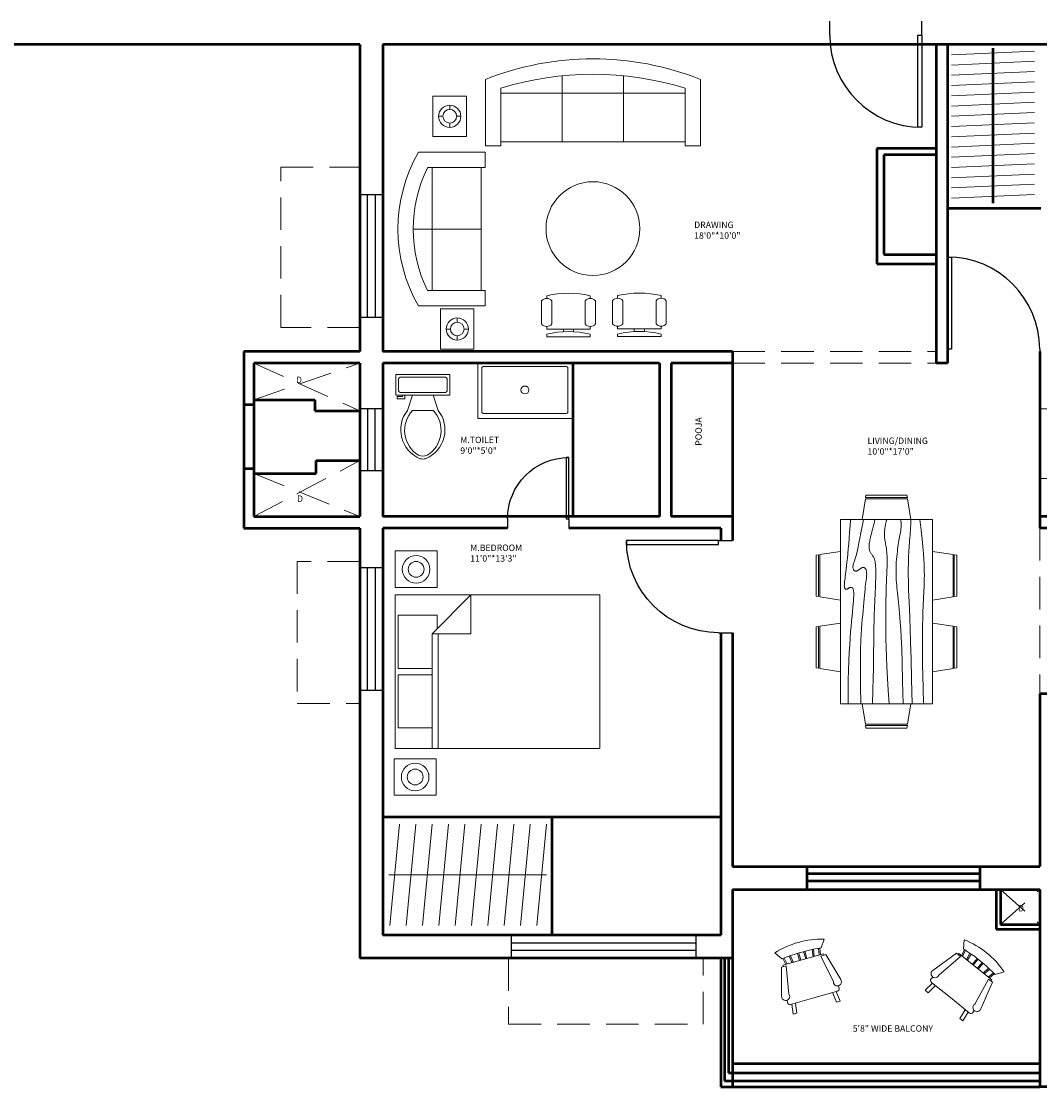
# Model space of a CAD drawing. Units: inches. Extents: x 291 to 2631, y 456 to 2623.
# Tile 7 of 22: x 1463 to 1861, y 515 to 931. Entities that reach past the tile are written whole.
import ezdxf

# ---------------------------------------------------------------- set-up
doc = ezdxf.new("R2010")
doc.units = ezdxf.units.IN
doc.linetypes.add('DASHED', pattern=[19.05, 12.7, -6.35])
for name, color, linetype, lineweight in [('A-ANNO-TEXT', 3, 'Continuous', 25), ('A-AREA-IDEN', 7, 'Continuous', 25), ('A-DOOR', 3, 'Continuous', 25), ('A-FLOR-FIXT', 9, 'Continuous', 18), ('A-FLOR-OVHD', 1, 'DASHED', 18), ('A-FURN', 8, 'Continuous', 18), ('A-GLAZ', 4, 'Continuous', 25), ('A-WALL', 7, 'Continuous', 50)]:
    doc.layers.add(name, color=color, linetype=linetype, lineweight=lineweight)
doc.styles.get("Standard").update_dxf_attribs({"font": 'arial.ttf'})

# ---------------------------------------------------------------- blocks, each defined once
blk = doc.blocks.new('*U2')
for p, q in [((0, 0), (0, -6)), ((40, 0), (40, -6))]:
    blk.add_line(p, q)
blk.add_lwpolyline([(0, 0), (0, 40), (1.75, 40), (1.75, 0)], close=True)
blk.add_arc((0, 0), 40, 0, 90)
blk = doc.blocks.new('Sofa - Roundback 7 ft.')
for p, q in [((-12.00002, -32.4421), (-12.00003, -6.5971)), ((11.99997, -32.4421), (11.99998, -6.5971)), ((-36.000027, -34), (-36.000027, -11.4696)), ((35.99998, -34), (35.99998, -11.4696)), ((-35.999844, -13.3819), (35.9998, -13.3819)), ((-36.000027, -32.4421), (35.99998, -32.4421))]:
    blk.add_line(p, q)
for points in [[(-36.000027, -34), (-42.000027, -34), (-42.000027, -8)], [(41.99998, -8), (41.99998, -34), (35.99998, -34)]]:
    blk.add_lwpolyline(points)
for centre, radius, start, end in [((0, -114.25), 114.25, 68.43141, 111.5686), ((-0.00001, -127.1968), 121.1968, 72.72033, 107.2797)]:
    blk.add_arc(centre, radius, start, end)
blk = doc.blocks.new('Sofa - Roundback Loveseat 5 ft.')
for p, q in [((0, -32.44198), (0, -5.99998)), ((-24, -33.99998), (-24, -11.46958)), ((24.00004, -33.99998), (24.00004, -11.46958)), ((-23.9998, -13.38178), (23.99986, -13.38178)), ((-24, -32.44198), (24.00004, -32.44198))]:
    blk.add_line(p, q)
for points in [[(-24, -33.99998), (-30, -33.99998), (-30, -7.99998)], [(30.00004, -7.99998), (30.00004, -33.99998), (24.00004, -33.99998)]]:
    blk.add_lwpolyline(points)
for centre, radius, start, end in [((0, -60.24998), 60.24998, 60.13715, 119.8628), ((0, -61.38438), 55.38444, 64.32083, 115.6792)]:
    blk.add_arc(centre, radius, start, end)
blk = doc.blocks.new('Chair - Desk')
for p, q in [((-8.5, 0), (-8.5, -1)), ((-8.5, 0), (8.5, 0)), ((8.5, 0), (8.5, -1)), ((-8.5, -3), (-8.5, -4)), ((-8.5, -3), (8.5, -3)), ((-2, -3), (-2, -1.9355)), ((2, -1.9576), (2, -3)), ((8.5, -3), (8.5, -4)), ((-10.5, -5), (-10.5, -14)), ((-6.5, -14), (-6.5, -5)), ((6.5, -5), (6.5, -14)), ((10.5, -14), (10.5, -5)), ((-8.5, -15), (-8.5, -16)), ((8.5, -15), (8.5, -16))]:
    blk.add_line(p, q)
for centre, radius, start, end in [((-8.5, -6.5), 2.5, 36.8699, 143.1301), ((0, 34.625), 36.625, 256.5803, 283.4197), ((8.5, -6.5), 2.5, 36.8699, 143.1301), ((-8.5, -12.5), 2.5, 216.8699, 323.1301), ((0, 19.625), 36.625, 256.5803, 283.4197), ((8.5, -12.5), 2.5, 216.8699, 323.1301)]:
    blk.add_arc(centre, radius, start, end)
blk = doc.blocks.new('Toilet - top')
for p, q in [((9.5, -6), (9.5, -2)), ((-8, -8.5), (-8, -8)), ((-7, -8), (-7, -9.5)), ((-4, -8), (-6, -14)), ((4, -8), (6, -14)), ((-10, -8.5), (-8, -8.5)), ((-10, -9.5), (-10, -8.5)), ((-7, -9.5), (-10, -9.5)), ((4, -14), (-4, -14))]:
    blk.add_line(p, q)
blk.add_lwpolyline([(10.5, -8), (10.5, 0), (-10.5, 0), (-10.5, -8)], close=True)
for points in [[(-9.5, -2), (-9.5, -6)], [(8.5, -1), (-8.5, -1)], [(-8.5, -7), (8.5, -7)]]:
    blk.add_lwpolyline(points)
for centre, radius, start, end in [((-8.62, -1.88), 0.884, 81.8699, 188.1301), ((8.62, -1.88), 0.884, 351.8699, 98.1301), ((-8.62, -6.12), 0.884, 171.8699, 278.1301), ((8.62, -6.12), 0.884, 261.8699, 8.1301), ((3.52, -21.58), 12.17, 141.4691, 247.9714), ((4.2, -21.82), 11.33, 136.3677, 238.9468), ((-3.52, -21.58), 12.17, 292.0284, 38.5307), ((-4.2, -21.82), 11.33, 301.053, 43.6321), ((0, -27.88), 4, 245.7318, 294.2682), ((0, -29), 4, 254.8605, 285.1395)]:
    blk.add_arc(centre, radius, start, end)
blk = doc.blocks.new('Bed - Queen')
for p, q in [((0, -80.00003), (0, 0)), ((0, 0), (59.99999, 0)), ((59.99999, 0), (59.99999, -80.00003)), ((7.99999, -1.2), (28.79998, -1.2)), ((7.99999, -14.4), (7.99999, -1.2)), ((28.79998, -1.2), (28.79998, -14.4)), ((31.19999, -1.2), (51.99999, -1.2)), ((31.19999, -14.4), (31.19999, -1.2)), ((51.99999, -1.2), (51.99999, -16.4)), ((0, -14.4), (44.8, -14.4)), ((59.99999, -29.6), (44.8, -14.4)), ((44.8, -14.4), (44.8, -29.6)), ((51.99999, -16.4), (46.79936, -16.4)), ((44.8, -16.8), (0, -16.8)), ((44.8, -29.6), (59.99999, -29.6)), ((59.99999, -80.00003), (0, -80.00003))]:
    blk.add_line(p, q)
blk = doc.blocks.new('Dining Set - 36 x 72 in.')
for p, q in [((-22.2343, 26.00059), (-23.4847, 17.99762)), ((-22.2304, 26), (-5.7608, 26)), ((-22, 27.5), (-22.1562, 26.50042)), ((-5.8416, 26.5), (-22.1534, 26.5)), ((-22, 27.5), (-6, 27.5)), ((-5.8437, 26.49966), (-6, 27.5)), ((-4.5152, 17.99762), (-5.7655, 25.99926)), ((5.7657, 26.00059), (4.5153, 17.99762)), ((5.7696, 26), (22.2392, 26)), ((6, 27.5), (5.8438, 26.50042)), ((22.1584, 26.5), (5.8466, 26.5)), ((6, 27.5), (22, 27.5)), ((22.1563, 26.49966), (22, 27.5)), ((23.4848, 17.99762), (22.2345, 25.99926)), ((36, 18), (-36, 18)), ((-36, 18), (-36, -18)), ((36, -18), (36, 18)), ((-44.0006, 8.23428), (-35.9976, 9.48474)), ((44.0006, 8.23428), (35.9976, 9.48474)), ((-45.5, 8), (-44.5004, 8.15617)), ((-45.5, 8), (-45.5, -8)), ((-44.5, -8.15843), (-44.5, 8.15338)), ((-44, 8.23041), (-44, -8.23915)), ((44, 8.23041), (44, -8.23915)), ((44.5, -8.15843), (44.5, 8.15338)), ((45.5, 8), (44.5005, 8.15617)), ((45.5, 8), (45.5, -8)), ((-44.4997, -8.15631), (-45.5, -8)), ((-35.9976, -9.48476), (-43.9993, -8.2345)), ((35.9976, -9.48476), (43.9993, -8.2345)), ((44.4997, -8.15631), (45.5, -8)), ((-36, -18), (36, -18)), ((-22.2343, -26.0006), (-23.4847, -17.99762)), ((-4.5152, -17.99762), (-5.7655, -25.99928)), ((5.7657, -26.0006), (4.5153, -17.99762)), ((23.4848, -17.99762), (22.2345, -25.99928)), ((-22.2304, -26), (-5.7608, -26)), ((-22, -27.5), (-22.1562, -26.50044)), ((-5.8416, -26.5), (-22.1534, -26.5)), ((-22, -27.5), (-6, -27.5)), ((-5.8437, -26.49967), (-6, -27.5)), ((5.7696, -26), (22.2392, -26)), ((6, -27.5), (5.8438, -26.50044)), ((22.1584, -26.5), (5.8466, -26.5)), ((6, -27.5), (22, -27.5)), ((22.1563, -26.49967), (22, -27.5))]:
    blk.add_line(p, q)
for points in [[(-36, 15), (-31.1772, 14.97754), (-26.8079, 14.91406), (-22.8538, 14.81543), (-19.276, 14.6875), (-16.0362, 14.53613), (-13.0957, 14.36718), (-10.4159, 14.18652), (-7.9583, 14), (-5.6904, 13.81315), (-3.6035, 13.63021), (-1.6954, 13.45508), (0.0365, 13.29166), (1.5945, 13.14388), (2.9811, 13.01562), (4.1988, 12.9108), (5.25, 12.83333), (6.1393, 12.78613), (6.8802, 12.76823), (7.4883, 12.77767), (7.9792, 12.8125), (8.3685, 12.87077), (8.6719, 12.95052), (8.9049, 13.0498), (9.0833, 13.16666), (9.2205, 13.29899), (9.3216, 13.44401), (9.3895, 13.59879), (9.4271, 13.76041), (9.4373, 13.92594), (9.4232, 14.09245), (9.3875, 14.257), (9.3333, 14.41666), (9.2638, 14.56917), (9.1836, 14.71484), (9.0975, 14.85465), (9.0104, 14.98958), (8.9272, 15.1206), (8.8529, 15.2487), (8.7922, 15.37483), (8.75, 15.5), (8.7305, 15.62467), (8.7344, 15.74739), (8.7617, 15.86621), (8.8125, 15.97916), (8.8867, 16.08431), (8.9844, 16.17968), (9.1055, 16.26334), (9.25, 16.33333), (9.4189, 16.38802), (9.6172, 16.42708), (9.8506, 16.45052), (10.125, 16.45833), (10.4463, 16.45052), (10.8203, 16.42708), (11.2529, 16.38802), (11.75, 16.33333), (12.3184, 16.26318), (12.9694, 16.17838), (13.7151, 16.07991), (14.5677, 15.96875), (15.5395, 15.84586), (16.6426, 15.71224), (17.8893, 15.56884), (19.2917, 15.41666), (20.859, 15.25667), (22.5879, 15.08984), (24.4721, 14.91715), (26.5052, 14.73958), (28.6809, 14.5581), (30.9929, 14.3737), (33.4347, 14.18733), (36, 14)], [(-36, 10), (-28.9766, 10.14274), (-23.1725, 10.20442), (-18.4241, 10.19775), (-14.5677, 10.13541), (-11.4399, 10.03011), (-8.877, 9.89453), (-6.7154, 9.74137), (-4.7917, 9.58333), (-2.9698, 9.43082), (-1.2246, 9.28515), (0.4415, 9.14534), (2.026, 9.01041), (3.5266, 8.87939), (4.9408, 8.7513), (6.266, 8.62516), (7.5, 8.5), (8.6411, 8.37549), (9.6914, 8.2539), (10.6538, 8.13818), (11.5312, 8.03125), (12.3267, 7.93603), (13.043, 7.85547), (13.6831, 7.79248), (14.25, 7.75), (14.7471, 7.7303), (15.1797, 7.73307), (15.5537, 7.75732), (15.875, 7.80208), (16.1494, 7.86637), (16.3828, 7.94922), (16.5811, 8.04964), (16.75, 8.16666), (16.8944, 8.29915), (17.0143, 8.44531), (17.1089, 8.60319), (17.1771, 8.77083), (17.218, 8.94629), (17.2305, 9.1276), (17.2137, 9.31282), (17.1667, 9.5), (17.0895, 9.6875), (16.987, 9.875), (16.8649, 10.0625), (16.7292, 10.25), (16.5856, 10.4375), (16.4401, 10.625), (16.2985, 10.8125), (16.1667, 11), (16.05, 11.18733), (15.9518, 11.3737), (15.8752, 11.5581), (15.8229, 11.73958), (15.798, 11.91715), (15.8034, 12.08984), (15.842, 12.25667), (15.9167, 12.41666), (16.0295, 12.56836), (16.1784, 12.70833), (16.3605, 12.83268), (16.5729, 12.9375), (16.8127, 13.01888), (17.0768, 13.07291), (17.3625, 13.0957), (17.6667, 13.08333), (17.9894, 13.03312), (18.3418, 12.94726), (18.7382, 12.82918), (19.1927, 12.68229), (19.7195, 12.51001), (20.3327, 12.31575), (21.0465, 12.10294), (21.875, 11.875), (22.8357, 11.63354), (23.959, 11.37304), (25.2786, 11.08618), (26.8282, 10.76562), (28.6414, 10.40405), (30.752, 9.99414), (33.1936, 9.52856), (36, 9)], [(-36, 5.5), (-30.7157, 5.3348), (-26.069, 5.20963), (-21.9946, 5.11767), (-18.4271, 5.05208), (-15.3009, 5.00602), (-12.5508, 4.97265), (-10.1112, 4.94515), (-7.9167, 4.91666), (-5.909, 4.88167), (-4.0586, 4.83984), (-2.3429, 4.79215), (-0.7396, 4.73958), (0.7739, 4.6831), (2.22, 4.6237), (3.6213, 4.56233), (5, 4.5), (6.373, 4.43782), (7.7344, 4.3776), (9.0723, 4.32129), (10.375, 4.27083), (11.6309, 4.22819), (12.8281, 4.19531), (13.9551, 4.17415), (15, 4.16666), (15.954, 4.17448), (16.819, 4.19791), (17.6001, 4.23698), (18.3021, 4.29166), (18.9299, 4.36198), (19.4883, 4.44791), (19.9823, 4.54948), (20.4167, 4.66666), (20.7969, 4.79899), (21.1302, 4.94401), (21.4245, 5.09879), (21.6875, 5.26041), (21.9271, 5.42594), (22.1511, 5.59245), (22.3672, 5.757), (22.5834, 5.91666), (22.8065, 6.06868), (23.0404, 6.21093), (23.2879, 6.34147), (23.5521, 6.45833), (23.8358, 6.55957), (24.142, 6.64323), (24.4735, 6.70735), (24.8334, 6.75), (25.2235, 6.76969), (25.642, 6.76692), (26.0858, 6.74267), (26.5521, 6.69791), (27.0379, 6.63362), (27.5404, 6.55078), (28.0565, 6.45036), (28.5834, 6.33333), (29.1242, 6.19987), (29.7071, 6.04687), (30.3661, 5.87044), (31.1354, 5.66666), (32.0493, 5.43164), (33.142, 5.16146), (34.4475, 4.85221), (36, 4.5)], [(-36, -1), (-30.7915, -0.6591), (-26.0195, -0.38216), (-21.6519, -0.16284), (-17.6563, 0.00521), (-14.0005, 0.12833), (-10.6523, 0.21289), (-7.5796, 0.26522), (-4.75, 0.29166), (-2.134, 0.29793), (0.2878, 0.28711), (2.5317, 0.26163), (4.6146, 0.22396), (6.5529, 0.17651), (8.3633, 0.12174), (10.0623, 0.06209), (11.6667, 0), (13.1899, -0.06201), (14.6341, -0.1211), (15.9982, -0.17432), (17.2813, -0.21875), (18.4823, -0.25147), (19.6003, -0.26953), (20.6343, -0.27002), (21.5834, -0.25), (22.4481, -0.20768), (23.2357, -0.14584), (23.9549, -0.06836), (24.6146, 0.02083), (25.2235, 0.11784), (25.7904, 0.21875), (26.3241, 0.31966), (26.8334, 0.41666), (27.3265, 0.50618), (27.8099, 0.58593), (28.2894, 0.65397), (28.7709, 0.70833), (29.2601, 0.74707), (29.763, 0.76823), (30.2855, 0.76985), (30.8334, 0.75), (31.4088, 0.70784), (31.9994, 0.64713), (32.589, 0.57275), (33.1615, 0.48958), (33.7008, 0.4025), (34.1908, 0.3164), (34.6153, 0.23616), (34.9584, 0.16666), (35.2099, 0.11165), (35.3848, 0.07031), (35.504, 0.04069), (35.5886, 0.02083), (35.6594, 0.00879), (35.7377, 0.0026), (35.8442, 0.00032), (36, 0)], [(-36, -6.5), (-27.1843, -6.31267), (-20.084, -6.1263), (-14.469, -5.9419), (-10.1094, -5.76042), (-6.7752, -5.58285), (-4.2363, -5.41016), (-2.2629, -5.24333), (-0.625, -5.08334), (0.8708, -4.93099), (2.2715, -4.78646), (3.5872, -4.64974), (4.8281, -4.52084), (6.0046, -4.39974), (7.127, -4.28646), (8.2053, -4.18099), (9.25, -4.08334), (10.2705, -3.99382), (11.2734, -3.91407), (12.2647, -3.84603), (13.25, -3.79167), (14.2354, -3.75293), (15.2266, -3.73177), (16.2295, -3.73015), (17.25, -3.75), (18.2912, -3.79248), (19.3451, -3.85547), (20.4009, -3.93604), (21.4479, -4.03125), (22.4754, -4.13819), (23.4727, -4.25391), (24.4289, -4.37549), (25.3334, -4.5), (26.1785, -4.62492), (26.9694, -4.74935), (27.7145, -4.87281), (28.4219, -4.99479), (29.1, -5.11483), (29.7572, -5.23242), (30.4016, -5.34709), (31.0417, -5.45834), (31.6837, -5.56437), (32.3262, -5.65821), (32.9658, -5.73153), (33.599, -5.77604), (34.2224, -5.78345), (34.8327, -5.74545), (35.4264, -5.65373), (36, -5.5)], [(-36, -10), (-26.4022, -9.81299), (-18.4675, -9.62891), (-11.9839, -9.45069), (-6.7396, -9.28125), (-2.5226, -9.12354), (0.8789, -8.98047), (3.6769, -8.85498), (6.0833, -8.75), (8.2767, -8.66765), (10.3021, -8.60677), (12.1712, -8.56543), (13.8958, -8.54167), (15.4876, -8.53353), (16.9583, -8.53907), (18.3197, -8.55632), (19.5834, -8.58334), (20.7616, -8.61841), (21.8685, -8.66081), (22.9188, -8.71004), (23.9271, -8.76563), (24.9081, -8.82707), (25.8763, -8.89388), (26.8465, -8.96558), (27.8334, -9.04167), (28.8474, -9.12118), (29.8828, -9.20117), (30.93, -9.27824), (31.9792, -9.34896), (33.0205, -9.40991), (34.0443, -9.45768), (35.0407, -9.48885), (36, -9.5)], [(-36, -14.5), (-30.0881, -14.33513), (-25.0332, -14.21224), (-20.7312, -14.12647), (-17.0781, -14.07292), (-13.97, -14.04671), (-11.3027, -14.04297), (-8.9724, -14.05681), (-6.875, -14.08334), (-4.9224, -14.11833), (-3.0905, -14.16016), (-1.3709, -14.20785), (0.2448, -14.26042), (1.7647, -14.3169), (3.1973, -14.3763), (4.5507, -14.43767), (5.8333, -14.5), (7.0554, -14.5621), (8.235, -14.62175), (9.3922, -14.67652), (10.5469, -14.72396), (11.7192, -14.76164), (12.929, -14.78711), (14.1965, -14.79794), (15.5417, -14.79167), (16.9933, -14.76424), (18.6152, -14.70508), (20.4804, -14.60197), (22.6615, -14.44271), (25.2312, -14.21509), (28.2624, -13.9069), (31.8277, -13.50594), (36, -13)]]:
    blk.add_lwpolyline(points)
blk = doc.blocks.new('Chair - Rocking')
for p, q in [((-8, -4.5), (-10, -1.5)), ((-1.5, -4.05012), (-1.5, -7)), ((-1, -7), (-1, -4.05012)), ((1, -7), (1, -4.04655)), ((1.5, -4.05012), (1.5, -7)), ((8, -4.5), (10, -1.5)), ((-9, -7.5), (-12, -18.49999)), ((-7, -7.5), (-9, -7.5)), ((-9, -18.49999), (-7, -7.5)), ((-8.23428, -6.99939), (-8.3093, -7.47958)), ((-8.23041, -7), (8.23915, -7)), ((-7.5, -4.5), (-7, -7)), ((-6.5, -7), (-7.02225, -4.43)), ((-4.5, -7), (-4.96674, -4.19951)), ((-4, -7), (-4.40532, -4.16272)), ((4, -7), (4.40187, -4.18694)), ((4.5, -7), (4.96761, -4.19437)), ((6.5, -7), (7, -4.4057)), ((7.5, -4.5), (7, -7)), ((7, -7.5), (9, -7.5)), ((9, -18.49999), (7, -7.5)), ((8.31071, -7.48854), (8.23449, -7.00073)), ((9, -7.5), (12, -18.49999)), ((-10.36644, -20.64523), (-10.5, -21.49999)), ((10.5, -21.49999), (10.3575, -20.58798)), ((-9, -22.49999), (-9.5, -26.49999)), ((0, -22.49999), (-9.5, -22.49999)), ((-8, -26.49999), (-7.5, -22.49999)), ((0, -22.49999), (9.5, -22.49999)), ((8, -26.49999), (7.5, -22.49999)), ((9, -22.49999), (9.5, -26.49999)), ((-9.5, -26.49999), (-8, -26.49999)), ((9.5, -26.49999), (8, -26.49999))]:
    blk.add_line(p, q)
for centre, radius, start, end in [((0, -34.08333), 34.08333, 72.93847, 107.0615), ((0, -68.25004), 64.25, 93.92211, 97.15267), ((0, -68.25004), 64.25, 82.84733, 93.92211), ((-10.5, -18.99999), 1.58114, 161.5651, 18.43495), ((10.5, -18.99999), 1.58114, 161.5651, 18.43495), ((-9.5, -21.49999), 1, 180, 270), ((9.5, -21.49999), 1, 270, 0)]:
    blk.add_arc(centre, radius, start, end)
blk = doc.blocks.new('WIN-1800')
for p, q in [((0, 9), (72, 9)), ((0, 0), (0, 9)), ((72, 9), (72, 0)), ((0, 6), (72, 6)), ((72, 3), (0, 3)), ((72, 0), (0, 0))]:
    blk.add_line(p, q)
blk = doc.blocks.new('WIN-1200')
for p, q in [((0, 0), (0, 48)), ((0, 48), (9, 48)), ((3, 0), (3, 48)), ((6, 48), (6, 0)), ((9, 48), (9, 0)), ((9, 0), (0, 0))]:
    blk.add_line(p, q)
blk = doc.blocks.new('WIN-600')
for p, q in [((24, 9), (0, 9)), ((0, 9), (0, 0)), ((24, 0), (24, 9)), ((24, 6), (0, 6)), ((0, 3), (24, 3)), ((0, 0), (24, 0))]:
    blk.add_line(p, q)
blk = doc.blocks.new('LAMP-A')
for p, q in [((6.55, 12.25), (6.55, 10.56)), ((2.2, 7.9), (3.88, 7.9)), ((6.55, 5.24), (6.55, 3.56)), ((9.21, 7.9), (10.89, 7.9))]:
    blk.add_line(p, q)
blk.add_lwpolyline([(0, 15.8), (13.09, 15.8), (13.09, 0), (0, 0)], close=True)
for radius in [4.34, 2.66]:
    blk.add_circle((6.55, 7.9), radius)

msp = doc.modelspace()

# ---------------------------------------------------------------- linework, layer by layer
at = {"layer": 'A-FLOR-OVHD'}
for p, q in [((1564.45, 811.41), (1564.45, 873.98)), ((1564.45, 873.98), (1595.37, 873.98)), ((1595.37, 811.41), (1564.45, 811.41)), ((1740.87, 801.98), (1820.37, 801.98)), ((1553.94, 797.48), (1595.37, 778.76)), ((1553.94, 783.11), (1595.37, 797.48)), ((1740.87, 797.48), (1820.37, 797.48)), ((1553.94, 737.48), (1595.37, 759.4)), ((1553.94, 754.3), (1595.37, 737.48)), ((1860.87, 732.98), (1860.87, 668.21)), ((1595.37, 720), (1570.9, 720)), ((1570.9, 720), (1570.9, 664.49)), ((1570.9, 664.49), (1595.37, 664.49)), ((1845.6, 591.78), (1860.87, 578.2)), ((1845.6, 578.2), (1860.87, 591.78)), ((1653.4, 564.98), (1653.4, 539.19)), ((1729.39, 539.19), (1729.39, 564.98)), ((1653.4, 539.19), (1729.39, 539.19))]:
    msp.add_line(p, q, dxfattribs=at)
at = {"layer": 'A-FURN'}
for p, q in [((1826.44, 917.89), (1858.82, 919.36)), ((1826.44, 913.89), (1858.82, 915.36)), ((1826.44, 909.89), (1858.82, 911.35)), ((1826.44, 905.88), (1858.82, 907.35)), ((1826.44, 901.88), (1858.82, 903.35)), ((1826.44, 897.88), (1858.82, 899.34)), ((1826.44, 893.88), (1858.82, 895.34)), ((1826.44, 889.87), (1858.82, 891.34)), ((1826.44, 885.87), (1858.82, 887.34)), ((1826.44, 881.87), (1858.82, 883.33)), ((1826.44, 877.86), (1858.82, 879.33)), ((1826.44, 873.86), (1858.82, 875.33)), ((1826.44, 869.86), (1858.82, 871.32)), ((1826.44, 865.86), (1858.82, 867.32)), ((1826.44, 861.85), (1858.82, 863.32)), ((1607.03, 577.73), (1610.81, 617.27)), ((1613.41, 577.73), (1617.18, 617.27)), ((1619.79, 577.73), (1623.56, 617.27)), ((1626.16, 577.73), (1629.94, 617.27)), ((1632.54, 577.73), (1636.31, 617.27)), ((1638.92, 577.73), (1642.69, 617.27)), ((1645.29, 577.73), (1649.07, 617.27)), ((1651.67, 577.73), (1655.44, 617.27)), ((1658.05, 577.73), (1661.82, 617.27)), ((1664.42, 577.73), (1668.2, 617.27)), ((1606.67, 597.5), (1668.21, 597.5))]:
    msp.add_line(p, q, dxfattribs=at)
for points in [[(1678.58, 797.48), (1641.42, 797.48), (1641.42, 775.82), (1678.58, 775.82)], [(1860.87, 779.65), (1880.37, 779.65), (1880.37, 752.33), (1860.87, 752.33)], [(1609.07, 724.05), (1625.55, 724.05), (1625.55, 709.75), (1609.07, 709.75)], [(1608.69, 642.92), (1625.17, 642.92), (1625.17, 628.62), (1608.69, 628.62)]]:
    msp.add_lwpolyline(points, close=True, dxfattribs=at)
msp.add_lwpolyline([(1643.5, 796.07), (1676.08, 796.07, -0.414214), (1676.58, 795.57), (1676.58, 778.32, -0.414214), (1676.08, 777.82), (1643.5, 777.82, -0.414214), (1643, 778.32), (1643, 795.57, -0.414214)], format="xyb", close=True, dxfattribs=at)
for centre, radius in [((1686.36, 849.98), 18.32), ((1659.79, 786.95), 1.55), ((1617.31, 716.9), 5.39), ((1617.31, 716.9), 3.08), ((1616.93, 635.77), 5.39), ((1616.93, 635.77), 3.08)]:
    msp.add_circle(centre, radius, dxfattribs=at)
at = {"layer": 'A-WALL'}
for p, q in [((1595.37, 921.98), (1418.5, 921.98)), ((1595.37, 921.98), (1595.37, 801.98)), ((1980.87, 921.98), (1604.37, 921.98)), ((1604.37, 921.98), (1604.37, 801.98)), ((1820.37, 921.98), (1820.37, 797.48)), ((1824.87, 921.98), (1824.87, 797.48)), ((1842.63, 920.47), (1842.63, 859.88)), ((1820.37, 881.26), (1797.23, 881.26)), ((1797.23, 881.26), (1797.23, 836.28)), ((1820.37, 878.82), (1799.97, 878.82)), ((1799.97, 878.82), (1799.97, 839.82)), ((1861.27, 857.84), (1824.87, 857.84)), ((1799.97, 839.82), (1820.37, 839.82)), ((1797.23, 836.28), (1820.37, 836.28)), ((1595.37, 801.98), (1549.99, 801.98)), ((1549.99, 801.98), (1549.99, 732.98)), ((1595.37, 801.98), (1549.99, 801.98)), ((1740.87, 801.98), (1604.37, 801.98)), ((1740.87, 801.98), (1740.87, 728.1)), ((1860.87, 801.98), (1860.87, 732.98)), ((1595.37, 797.48), (1553.94, 797.48)), ((1553.94, 797.48), (1553.94, 737.48)), ((1595.37, 797.48), (1595.37, 737.48)), ((1604.37, 797.48), (1604.37, 737.48)), ((1712.37, 797.48), (1604.37, 797.48)), ((1678.58, 797.48), (1678.58, 737.48)), ((1712.37, 797.48), (1712.37, 737.48)), ((1716.87, 797.48), (1716.87, 737.48)), ((1740.87, 797.48), (1716.87, 797.48)), ((1824.87, 797.48), (1820.37, 797.48)), ((1553.94, 783.11), (1577.77, 783.11)), ((1577.77, 783.11), (1577.77, 778.76)), ((1553.94, 781.11), (1549.99, 781.11)), ((1577.77, 778.76), (1595.37, 778.76)), ((1578.3, 754.3), (1578.3, 759.4)), ((1578.3, 759.4), (1595.37, 759.4)), ((1553.94, 756.12), (1549.99, 756.12)), ((1553.94, 754.3), (1578.3, 754.3)), ((1553.94, 737.48), (1595.37, 737.48)), ((1712.37, 737.48), (1604.37, 737.48)), ((1740.87, 737.48), (1716.87, 737.48)), ((1880.37, 737.48), (1860.87, 737.48)), ((1549.99, 732.98), (1595.37, 732.98)), ((1595.37, 732.98), (1595.37, 564.98)), ((1604.37, 732.98), (1604.37, 573.98)), ((1653.02, 732.98), (1604.37, 732.98)), ((1736.37, 732.98), (1677.02, 732.98)), ((1736.37, 732.98), (1736.37, 728.1)), ((1980.87, 732.98), (1860.87, 732.98)), ((1736.37, 692.1), (1736.37, 573.98)), ((1740.87, 692.1), (1740.87, 600.78)), ((1882.34, 668.21), (1860.87, 668.21)), ((1860.87, 668.21), (1860.87, 600.78)), ((1604.37, 620.14), (1736.37, 620.14)), ((1670.37, 620.14), (1670.37, 573.98)), ((1740.87, 600.78), (1860.87, 600.78)), ((1769.93, 600.78), (1769.93, 591.78)), ((1837.43, 600.78), (1837.43, 591.78)), ((1769.93, 598.06), (1837.43, 598.06)), ((1769.93, 595.19), (1837.43, 595.19)), ((1740.87, 591.78), (1860.87, 591.78)), ((1740.87, 591.78), (1740.87, 564.98)), ((1843.83, 591.78), (1843.83, 576.37)), ((1845.6, 591.78), (1845.6, 578.2)), ((1860.87, 591.78), (1860.87, 564.98)), ((1843.83, 576.37), (1860.87, 576.37)), ((1845.6, 578.2), (1860.87, 578.2)), ((1736.37, 573.98), (1604.37, 573.98)), ((1740.87, 564.98), (1595.37, 564.98)), ((1736.37, 564.98), (1736.37, 514.78)), ((1737.75, 564.98), (1737.75, 517.1)), ((1739.35, 564.98), (1739.35, 520.16)), ((1740.87, 564.98), (1740.87, 514.78)), ((1860.87, 564.98), (1860.87, 514.78)), ((1740.87, 523.78), (1860.87, 523.78)), ((1737.75, 517.1), (1860.87, 517.1)), ((1739.35, 520.16), (1860.87, 520.16)), ((1736.37, 514.78), (1740.87, 514.78)), ((1740.87, 514.78), (1860.87, 514.78)), ((1865.37, 514.78), (1860.87, 514.78))]:
    msp.add_line(p, q, dxfattribs=at)

# ---------------------------------------------------------------- block references
at = {"layer": 'A-DOOR', "yscale": 0.9, "zscale": 0.9}
for p, xscale, rotation in [((1814.85, 925.58), 0.9, 180), ((1735.47, 728.1), -0.9, 90)]:
    msp.add_blockref('*U2', p, dxfattribs=dict(at, xscale=xscale, rotation=rotation))
at = {"layer": 'A-DOOR'}
for p, xscale, yscale, zscale in [((1824.87, 802.88), 0.9, 0.9, 0.9), ((1677.02, 736.58), -0.6, 0.6, 0.6)]:
    msp.add_blockref('*U2', p, dxfattribs=dict(at, xscale=xscale, yscale=yscale, zscale=zscale))
at = {"layer": 'A-FLOR-FIXT'}
msp.add_blockref('Toilet - top', (1619.94, 792.96), dxfattribs=at)
at = {"layer": 'A-FURN'}
for name, p in [('Sofa - Roundback 7 ft.', (1686.36, 916.3)), ('LAMP-A', (1623.9, 885.99)), ('LAMP-A', (1626.82, 802.87))]:
    msp.add_blockref(name, p, dxfattribs=at)
for name, p, rotation in [('Sofa - Roundback Loveseat 5 ft.', (1610.22, 849.8), 90), ('Chair - Desk', (1676.83, 807.75), 180), ('Chair - Desk', (1704.53, 807.82), 180), ('Dining Set - 36 x 72 in.', (1801.02, 700.39), 90), ('Bed - Queen', (1609.13, 646.92), 90), ('Chair - Rocking', (1766.61, 571.16), 15.67595765379025), ('Chair - Rocking', (1840.12, 567.08), 321.0741999402937)]:
    msp.add_blockref(name, p, dxfattribs=dict(at, rotation=rotation))
at = {"layer": 'A-GLAZ'}
for name, p, rotation in [('WIN-1200', (1604.37, 863.3), 180), ('WIN-600', (1595.37, 779.55), 269.9999999999998), ('WIN-1200', (1604.37, 717.58), 180)]:
    msp.add_blockref(name, p, dxfattribs=dict(at, rotation=rotation))
msp.add_blockref('WIN-1800', (1654.57, 564.98), dxfattribs=at)

# ---------------------------------------------------------------- texts
at = {"layer": 'A-ANNO-TEXT', "char_height": 2.5, "attachment_point": 1}
for width, insert in [(3.177, (1570.39, 792.16)), (2.74, (1570.8, 745.73)), (1.7344, (1852.4, 585.73))]:
    msp.add_mtext_dynamic_manual_height_columns('D', width=width, gutter_width=12.5, heights=[0], dxfattribs=dict(at, insert=insert))
at = {"layer": 'A-AREA-IDEN', "char_height": 2.5, "attachment_point": 1}
for s, width, insert in [('DRAWING\\P18\'0"*10\'0"', 67.7604, (1725.91, 852.7)), ('M.TOILET\\P9\'0"*5\'0"', 28.0989, (1634.56, 768.68)), ('LIVING/DINING\\P10\'0"*17\'0"', 71.3719, (1793.61, 768.37)), ('M.BEDROOM\\P11\'0"*13\'3"', 49.5115, (1638.44, 726.57)), ('5\'8" WIDE BALCONY', 49.6481, (1787.85, 538.77))]:
    msp.add_mtext_dynamic_manual_height_columns(s, width=width, gutter_width=12.5, heights=[0], dxfattribs=dict(at, insert=insert))
at = {"layer": 'A-AREA-IDEN', "insert": (1726.39, 765.17), "char_height": 2.5, "attachment_point": 1, "rotation": 90}
msp.add_mtext_dynamic_manual_height_columns('POOJA', width=19.3787, gutter_width=12.5, heights=[0], dxfattribs=at)

doc.saveas('drawing.dxf')
